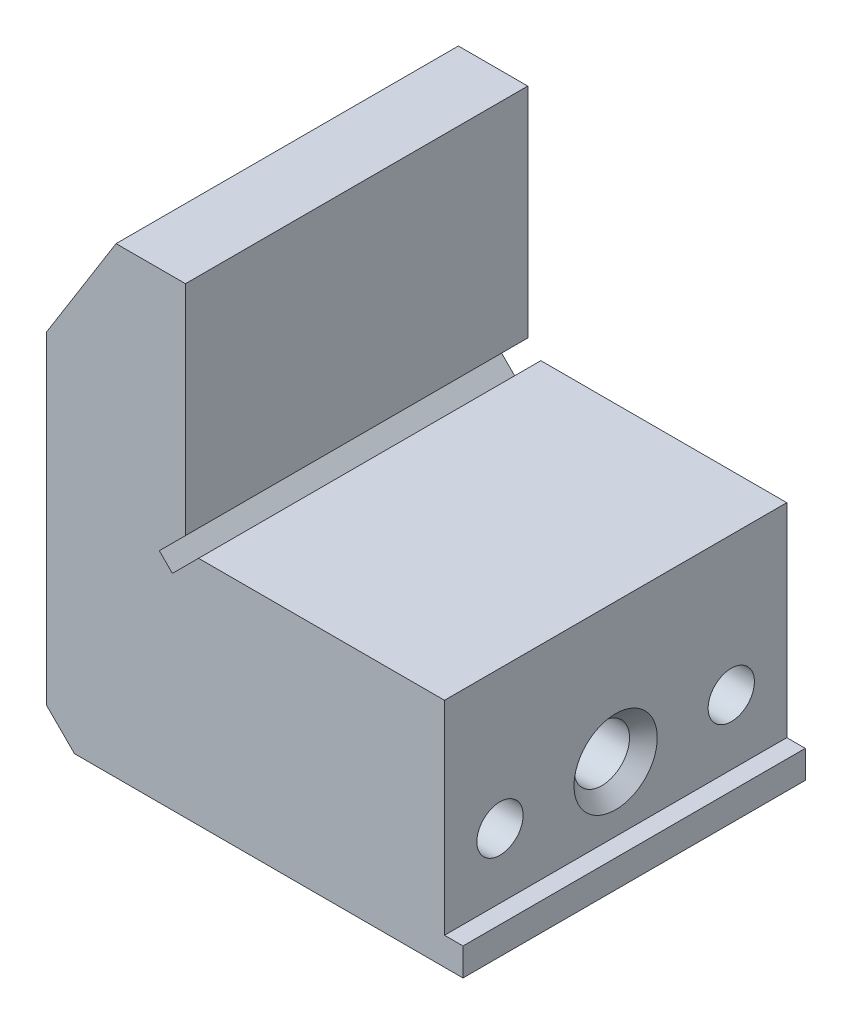
ISO-10303-21;
HEADER;
FILE_DESCRIPTION(('STEP AP214'),'2;1');
FILE_NAME('part.step','',(''),(''),'','','');
FILE_SCHEMA(('AUTOMOTIVE_DESIGN { 1 0 10303 214 1 1 1 1 }'));
ENDSEC;
DATA;
#1=APPLICATION_CONTEXT('core data for automotive mechanical design processes');
#2=APPLICATION_PROTOCOL_DEFINITION('international standard','automotive_design',2000,#1);
#3=PRODUCT_CONTEXT('',#1,'mechanical');
#4=PRODUCT('Part','Part','',(#3));
#5=PRODUCT_RELATED_PRODUCT_CATEGORY('part','',(#4));
#6=PRODUCT_DEFINITION_FORMATION('','',#4);
#7=PRODUCT_DEFINITION_CONTEXT('part definition',#1,'design');
#8=PRODUCT_DEFINITION('design','',#6,#7);
#9=PRODUCT_DEFINITION_SHAPE('','',#8);
#10=(LENGTH_UNIT() NAMED_UNIT(*) SI_UNIT(.MILLI.,.METRE.));
#11=(NAMED_UNIT(*) PLANE_ANGLE_UNIT() SI_UNIT($,.RADIAN.));
#12=(NAMED_UNIT(*) SI_UNIT($,.STERADIAN.) SOLID_ANGLE_UNIT());
#13=UNCERTAINTY_MEASURE_WITH_UNIT(LENGTH_MEASURE(1.E-05),#10,'distance_accuracy_value','');
#14=(GEOMETRIC_REPRESENTATION_CONTEXT(3) GLOBAL_UNCERTAINTY_ASSIGNED_CONTEXT((#13)) GLOBAL_UNIT_ASSIGNED_CONTEXT((#10,
#11,#12)) REPRESENTATION_CONTEXT('',''));
#15=CARTESIAN_POINT('',(0.,0.,0.));
#16=DIRECTION('',(0.,0.,1.));
#17=DIRECTION('',(1.,0.,0.));
#18=AXIS2_PLACEMENT_3D('',#15,#16,#17);
#19=CARTESIAN_POINT('',(3.,-25.,18.5));
#20=DIRECTION('',(0.707106781186548,0.707106781186547,0.));
#21=DIRECTION('',(0.,0.,-1.));
#22=AXIS2_PLACEMENT_3D('',#19,#20,#21);
#23=PLANE('',#22);
#24=DIRECTION('',(-0.707106781186547,0.707106781186548,0.));
#25=VECTOR('',#24,1.);
#26=CARTESIAN_POINT('',(3.00000000000001,-25.,-12.));
#27=LINE('',#26,#25);
#28=CARTESIAN_POINT('',(0.,-22.,-12.));
#29=VERTEX_POINT('',#28);
#30=CARTESIAN_POINT('',(3.00000000000001,-25.,-12.));
#31=VERTEX_POINT('',#30);
#32=EDGE_CURVE('E12',#29,#31,#27,.F.);
#33=ORIENTED_EDGE('',*,*,#32,.F.);
#34=DIRECTION('',(0.,0.,1.));
#35=VECTOR('',#34,1.);
#36=CARTESIAN_POINT('',(0.,-22.,18.5));
#37=LINE('',#36,#35);
#38=CARTESIAN_POINT('',(0.,-22.,-18.5));
#39=VERTEX_POINT('',#38);
#40=EDGE_CURVE('E318',#39,#29,#37,.T.);
#41=ORIENTED_EDGE('',*,*,#40,.F.);
#42=DIRECTION('',(0.707106781186547,-0.707106781186548,0.));
#43=VECTOR('',#42,1.);
#44=CARTESIAN_POINT('',(-11.,-11.,-18.5));
#45=LINE('',#44,#43);
#46=CARTESIAN_POINT('',(3.00000000000002,-25.,-18.5));
#47=VERTEX_POINT('',#46);
#48=EDGE_CURVE('E312',#47,#39,#45,.F.);
#49=ORIENTED_EDGE('',*,*,#48,.F.);
#50=DIRECTION('',(0.,0.,-1.));
#51=VECTOR('',#50,1.);
#52=CARTESIAN_POINT('',(3.,-25.,18.5));
#53=LINE('',#52,#51);
#54=EDGE_CURVE('E313',#31,#47,#53,.T.);
#55=ORIENTED_EDGE('',*,*,#54,.F.);
#56=EDGE_LOOP('',(#33,#41,#49,#55));
#57=FACE_BOUND('',#56,.T.);
#58=ADVANCED_FACE('F43',(#57),#23,.F.);
#59=CARTESIAN_POINT('',(45.,-25.,18.5));
#60=DIRECTION('',(0.,1.,0.));
#61=DIRECTION('',(-1.,0.,0.));
#62=AXIS2_PLACEMENT_3D('',#59,#60,#61);
#63=PLANE('',#62);
#64=DIRECTION('',(0.,0.,-1.));
#65=VECTOR('',#64,1.);
#66=CARTESIAN_POINT('',(27.,-25.,-12.));
#67=LINE('',#66,#65);
#68=CARTESIAN_POINT('',(27.,-25.,12.));
#69=VERTEX_POINT('',#68);
#70=CARTESIAN_POINT('',(27.,-25.,-12.));
#71=VERTEX_POINT('',#70);
#72=EDGE_CURVE('E206',#69,#71,#67,.T.);
#73=ORIENTED_EDGE('',*,*,#72,.T.);
#74=DIRECTION('',(-1.,0.,0.));
#75=VECTOR('',#74,1.);
#76=CARTESIAN_POINT('',(75.,-25.,-12.));
#77=LINE('',#76,#75);
#78=EDGE_CURVE('E204',#71,#31,#77,.T.);
#79=ORIENTED_EDGE('',*,*,#78,.T.);
#80=ORIENTED_EDGE('',*,*,#54,.T.);
#81=DIRECTION('',(1.,0.,0.));
#82=VECTOR('',#81,1.);
#83=CARTESIAN_POINT('',(45.,-25.,-18.5));
#84=LINE('',#83,#82);
#85=CARTESIAN_POINT('',(45.,-25.,-18.5));
#86=VERTEX_POINT('',#85);
#87=EDGE_CURVE('E245',#47,#86,#84,.T.);
#88=ORIENTED_EDGE('',*,*,#87,.T.);
#89=DIRECTION('',(0.,0.,-1.));
#90=VECTOR('',#89,1.);
#91=CARTESIAN_POINT('',(45.,-25.,18.5));
#92=LINE('',#91,#90);
#93=CARTESIAN_POINT('',(45.,-25.,18.5));
#94=VERTEX_POINT('',#93);
#95=EDGE_CURVE('E306',#94,#86,#92,.T.);
#96=ORIENTED_EDGE('',*,*,#95,.F.);
#97=DIRECTION('',(1.,0.,0.));
#98=VECTOR('',#97,1.);
#99=CARTESIAN_POINT('',(45.,-25.,18.5));
#100=LINE('',#99,#98);
#101=CARTESIAN_POINT('',(3.00000000000002,-25.,18.5));
#102=VERTEX_POINT('',#101);
#103=EDGE_CURVE('E251',#102,#94,#100,.T.);
#104=ORIENTED_EDGE('',*,*,#103,.F.);
#105=CARTESIAN_POINT('',(3.,-25.,12.));
#106=VERTEX_POINT('',#105);
#107=EDGE_CURVE('E315',#102,#106,#53,.T.);
#108=ORIENTED_EDGE('',*,*,#107,.T.);
#109=DIRECTION('',(-1.,0.,0.));
#110=VECTOR('',#109,1.);
#111=CARTESIAN_POINT('',(75.,-25.,12.));
#112=LINE('',#111,#110);
#113=EDGE_CURVE('E58',#69,#106,#112,.T.);
#114=ORIENTED_EDGE('',*,*,#113,.F.);
#115=EDGE_LOOP('',(#73,#79,#80,#88,#96,#104,#108,#114));
#116=FACE_BOUND('',#115,.T.);
#117=ADVANCED_FACE('F336',(#116),#63,.F.);
#118=CARTESIAN_POINT('',(45.,-22.,18.5));
#119=DIRECTION('',(-1.,0.,0.));
#120=DIRECTION('',(0.,0.,1.));
#121=AXIS2_PLACEMENT_3D('',#118,#119,#120);
#122=PLANE('',#121);
#123=DIRECTION('',(0.,1.,0.));
#124=VECTOR('',#123,1.);
#125=CARTESIAN_POINT('',(45.,-22.,-18.5));
#126=LINE('',#125,#124);
#127=CARTESIAN_POINT('',(45.,-22.,-18.5));
#128=VERTEX_POINT('',#127);
#129=EDGE_CURVE('E273',#86,#128,#126,.T.);
#130=ORIENTED_EDGE('',*,*,#129,.T.);
#131=DIRECTION('',(0.,0.,-1.));
#132=VECTOR('',#131,1.);
#133=CARTESIAN_POINT('',(45.,-22.,18.5));
#134=LINE('',#133,#132);
#135=CARTESIAN_POINT('',(45.,-22.,18.5));
#136=VERTEX_POINT('',#135);
#137=EDGE_CURVE('E303',#136,#128,#134,.T.);
#138=ORIENTED_EDGE('',*,*,#137,.F.);
#139=DIRECTION('',(0.,1.,0.));
#140=VECTOR('',#139,1.);
#141=CARTESIAN_POINT('',(45.,-22.,18.5));
#142=LINE('',#141,#140);
#143=EDGE_CURVE('E258',#94,#136,#142,.T.);
#144=ORIENTED_EDGE('',*,*,#143,.F.);
#145=ORIENTED_EDGE('',*,*,#95,.T.);
#146=EDGE_LOOP('',(#130,#138,#144,#145));
#147=FACE_BOUND('',#146,.T.);
#148=ADVANCED_FACE('F347',(#147),#122,.F.);
#149=CARTESIAN_POINT('',(43.,-22.,18.5));
#150=DIRECTION('',(0.,-1.,0.));
#151=DIRECTION('',(0.,0.,-1.));
#152=AXIS2_PLACEMENT_3D('',#149,#150,#151);
#153=PLANE('',#152);
#154=DIRECTION('',(-1.,0.,0.));
#155=VECTOR('',#154,1.);
#156=CARTESIAN_POINT('',(43.,-22.,-18.5));
#157=LINE('',#156,#155);
#158=CARTESIAN_POINT('',(43.,-22.,-18.5));
#159=VERTEX_POINT('',#158);
#160=EDGE_CURVE('E277',#128,#159,#157,.T.);
#161=ORIENTED_EDGE('',*,*,#160,.T.);
#162=DIRECTION('',(0.,0.,-1.));
#163=VECTOR('',#162,1.);
#164=CARTESIAN_POINT('',(43.,-22.,18.5));
#165=LINE('',#164,#163);
#166=CARTESIAN_POINT('',(43.,-22.,18.5));
#167=VERTEX_POINT('',#166);
#168=EDGE_CURVE('E304',#167,#159,#165,.T.);
#169=ORIENTED_EDGE('',*,*,#168,.F.);
#170=DIRECTION('',(-1.,0.,0.));
#171=VECTOR('',#170,1.);
#172=CARTESIAN_POINT('',(43.,-22.,18.5));
#173=LINE('',#172,#171);
#174=EDGE_CURVE('E256',#136,#167,#173,.T.);
#175=ORIENTED_EDGE('',*,*,#174,.F.);
#176=ORIENTED_EDGE('',*,*,#137,.T.);
#177=EDGE_LOOP('',(#161,#169,#175,#176));
#178=FACE_BOUND('',#177,.T.);
#179=ADVANCED_FACE('F354',(#178),#153,.F.);
#180=CARTESIAN_POINT('',(43.,0.,18.5));
#181=DIRECTION('',(-1.,0.,0.));
#182=DIRECTION('',(0.,0.,1.));
#183=AXIS2_PLACEMENT_3D('',#180,#181,#182);
#184=PLANE('',#183);
#185=CARTESIAN_POINT('',(43.,-15.,-12.5));
#186=DIRECTION('',(1.,0.,0.));
#187=DIRECTION('',(0.,0.,-1.));
#188=AXIS2_PLACEMENT_3D('',#185,#186,#187);
#189=CIRCLE('',#188,2.49999999999999);
#190=CARTESIAN_POINT('',(43.,-15.,-15.));
#191=VERTEX_POINT('',#190);
#192=EDGE_CURVE('E183',#191,#191,#189,.T.);
#193=ORIENTED_EDGE('',*,*,#192,.F.);
#194=EDGE_LOOP('',(#193));
#195=FACE_BOUND('',#194,.T.);
#196=CARTESIAN_POINT('',(43.,-15.,12.5));
#197=DIRECTION('',(1.,0.,0.));
#198=DIRECTION('',(0.,0.,-1.));
#199=AXIS2_PLACEMENT_3D('',#196,#197,#198);
#200=CIRCLE('',#199,2.49999999999999);
#201=CARTESIAN_POINT('',(43.,-15.,10.));
#202=VERTEX_POINT('',#201);
#203=EDGE_CURVE('E184',#202,#202,#200,.T.);
#204=ORIENTED_EDGE('',*,*,#203,.F.);
#205=EDGE_LOOP('',(#204));
#206=FACE_BOUND('',#205,.T.);
#207=CARTESIAN_POINT('',(43.,-15.,0.));
#208=DIRECTION('',(1.,0.,0.));
#209=DIRECTION('',(0.,0.,-1.));
#210=AXIS2_PLACEMENT_3D('',#207,#208,#209);
#211=CIRCLE('',#210,4.5);
#212=CARTESIAN_POINT('',(43.,-15.,-4.5));
#213=VERTEX_POINT('',#212);
#214=EDGE_CURVE('E193',#213,#213,#211,.T.);
#215=ORIENTED_EDGE('',*,*,#214,.F.);
#216=EDGE_LOOP('',(#215));
#217=FACE_BOUND('',#216,.T.);
#218=DIRECTION('',(0.,1.,0.));
#219=VECTOR('',#218,1.);
#220=CARTESIAN_POINT('',(43.,0.,-18.5));
#221=LINE('',#220,#219);
#222=CARTESIAN_POINT('',(43.,0.,-18.5));
#223=VERTEX_POINT('',#222);
#224=EDGE_CURVE('E279',#159,#223,#221,.T.);
#225=ORIENTED_EDGE('',*,*,#224,.T.);
#226=DIRECTION('',(0.,0.,-1.));
#227=VECTOR('',#226,1.);
#228=CARTESIAN_POINT('',(43.,0.,18.5));
#229=LINE('',#228,#227);
#230=CARTESIAN_POINT('',(43.,0.,18.5));
#231=VERTEX_POINT('',#230);
#232=EDGE_CURVE('E300',#231,#223,#229,.T.);
#233=ORIENTED_EDGE('',*,*,#232,.F.);
#234=DIRECTION('',(0.,1.,0.));
#235=VECTOR('',#234,1.);
#236=CARTESIAN_POINT('',(43.,0.,18.5));
#237=LINE('',#236,#235);
#238=EDGE_CURVE('E257',#167,#231,#237,.T.);
#239=ORIENTED_EDGE('',*,*,#238,.F.);
#240=ORIENTED_EDGE('',*,*,#168,.T.);
#241=EDGE_LOOP('',(#225,#233,#239,#240));
#242=FACE_BOUND('',#241,.T.);
#243=ADVANCED_FACE('F357',(#195,#206,#217,#242),#184,.F.);
#244=CARTESIAN_POINT('',(15.,0.,18.5));
#245=DIRECTION('',(0.,-1.,0.));
#246=DIRECTION('',(0.,0.,-1.));
#247=AXIS2_PLACEMENT_3D('',#244,#245,#246);
#248=PLANE('',#247);
#249=DIRECTION('',(-1.,0.,0.));
#250=VECTOR('',#249,1.);
#251=CARTESIAN_POINT('',(15.,0.,-18.5));
#252=LINE('',#251,#250);
#253=CARTESIAN_POINT('',(16.4142135623731,0.,-18.5));
#254=VERTEX_POINT('',#253);
#255=EDGE_CURVE('E278',#223,#254,#252,.T.);
#256=ORIENTED_EDGE('',*,*,#255,.T.);
#257=DIRECTION('',(0.,0.,1.));
#258=VECTOR('',#257,1.);
#259=CARTESIAN_POINT('',(16.4142135623731,0.,-18.5));
#260=LINE('',#259,#258);
#261=CARTESIAN_POINT('',(16.4142135623731,0.,18.5));
#262=VERTEX_POINT('',#261);
#263=EDGE_CURVE('E70',#254,#262,#260,.T.);
#264=ORIENTED_EDGE('',*,*,#263,.T.);
#265=DIRECTION('',(-1.,0.,0.));
#266=VECTOR('',#265,1.);
#267=CARTESIAN_POINT('',(15.,0.,18.5));
#268=LINE('',#267,#266);
#269=EDGE_CURVE('E265',#231,#262,#268,.T.);
#270=ORIENTED_EDGE('',*,*,#269,.F.);
#271=ORIENTED_EDGE('',*,*,#232,.T.);
#272=EDGE_LOOP('',(#256,#264,#270,#271));
#273=FACE_BOUND('',#272,.T.);
#274=ADVANCED_FACE('F358',(#273),#248,.F.);
#275=CARTESIAN_POINT('',(15.,25.,18.5));
#276=DIRECTION('',(-1.,0.,0.));
#277=DIRECTION('',(0.,-1.,0.));
#278=AXIS2_PLACEMENT_3D('',#275,#276,#277);
#279=PLANE('',#278);
#280=DIRECTION('',(0.,1.,0.));
#281=VECTOR('',#280,1.);
#282=CARTESIAN_POINT('',(15.,25.,18.5));
#283=LINE('',#282,#281);
#284=CARTESIAN_POINT('',(15.,1.4142135623731,18.5));
#285=VERTEX_POINT('',#284);
#286=CARTESIAN_POINT('',(15.,25.,18.5));
#287=VERTEX_POINT('',#286);
#288=EDGE_CURVE('E264',#285,#287,#283,.T.);
#289=ORIENTED_EDGE('',*,*,#288,.F.);
#290=DIRECTION('',(0.,0.,1.));
#291=VECTOR('',#290,1.);
#292=CARTESIAN_POINT('',(15.,1.4142135623731,-18.5));
#293=LINE('',#292,#291);
#294=CARTESIAN_POINT('',(15.,1.4142135623731,-18.5));
#295=VERTEX_POINT('',#294);
#296=EDGE_CURVE('E241',#295,#285,#293,.T.);
#297=ORIENTED_EDGE('',*,*,#296,.F.);
#298=DIRECTION('',(0.,1.,0.));
#299=VECTOR('',#298,1.);
#300=CARTESIAN_POINT('',(15.,25.,-18.5));
#301=LINE('',#300,#299);
#302=CARTESIAN_POINT('',(15.,25.,-18.5));
#303=VERTEX_POINT('',#302);
#304=EDGE_CURVE('E282',#295,#303,#301,.T.);
#305=ORIENTED_EDGE('',*,*,#304,.T.);
#306=DIRECTION('',(0.,0.,-1.));
#307=VECTOR('',#306,1.);
#308=CARTESIAN_POINT('',(15.,25.,18.5));
#309=LINE('',#308,#307);
#310=EDGE_CURVE('E298',#287,#303,#309,.T.);
#311=ORIENTED_EDGE('',*,*,#310,.F.);
#312=EDGE_LOOP('',(#289,#297,#305,#311));
#313=FACE_BOUND('',#312,.T.);
#314=ADVANCED_FACE('F373',(#313),#279,.F.);
#315=CARTESIAN_POINT('',(7.49843222291195,25.,18.5));
#316=DIRECTION('',(0.,-1.,0.));
#317=DIRECTION('',(0.,0.,-1.));
#318=AXIS2_PLACEMENT_3D('',#315,#316,#317);
#319=PLANE('',#318);
#320=DIRECTION('',(-1.,0.,0.));
#321=VECTOR('',#320,1.);
#322=CARTESIAN_POINT('',(7.49843222291195,25.,-18.5));
#323=LINE('',#322,#321);
#324=CARTESIAN_POINT('',(7.49843222291195,25.,-18.5));
#325=VERTEX_POINT('',#324);
#326=EDGE_CURVE('E281',#303,#325,#323,.T.);
#327=ORIENTED_EDGE('',*,*,#326,.T.);
#328=DIRECTION('',(0.,0.,-1.));
#329=VECTOR('',#328,1.);
#330=CARTESIAN_POINT('',(7.49843222291195,25.,18.5));
#331=LINE('',#330,#329);
#332=CARTESIAN_POINT('',(7.49843222291195,25.,18.5));
#333=VERTEX_POINT('',#332);
#334=EDGE_CURVE('E291',#333,#325,#331,.T.);
#335=ORIENTED_EDGE('',*,*,#334,.F.);
#336=DIRECTION('',(-1.,0.,0.));
#337=VECTOR('',#336,1.);
#338=CARTESIAN_POINT('',(7.49843222291195,25.,18.5));
#339=LINE('',#338,#337);
#340=EDGE_CURVE('E270',#287,#333,#339,.T.);
#341=ORIENTED_EDGE('',*,*,#340,.F.);
#342=ORIENTED_EDGE('',*,*,#310,.T.);
#343=EDGE_LOOP('',(#327,#335,#341,#342));
#344=FACE_BOUND('',#343,.T.);
#345=ADVANCED_FACE('F377',(#344),#319,.F.);
#346=CARTESIAN_POINT('',(0.,13.,18.5));
#347=DIRECTION('',(0.848048096156426,-0.529919264233206,0.));
#348=DIRECTION('',(0.529919264233206,0.848048096156425,0.));
#349=AXIS2_PLACEMENT_3D('',#346,#347,#348);
#350=PLANE('',#349);
#351=DIRECTION('',(-0.529919264233206,-0.848048096156425,0.));
#352=VECTOR('',#351,1.);
#353=CARTESIAN_POINT('',(0.,13.,-18.5));
#354=LINE('',#353,#352);
#355=CARTESIAN_POINT('',(0.,13.,-18.5));
#356=VERTEX_POINT('',#355);
#357=EDGE_CURVE('E289',#325,#356,#354,.T.);
#358=ORIENTED_EDGE('',*,*,#357,.T.);
#359=DIRECTION('',(0.,0.,-1.));
#360=VECTOR('',#359,1.);
#361=CARTESIAN_POINT('',(0.,13.,18.5));
#362=LINE('',#361,#360);
#363=CARTESIAN_POINT('',(0.,13.,18.5));
#364=VERTEX_POINT('',#363);
#365=EDGE_CURVE('E275',#364,#356,#362,.T.);
#366=ORIENTED_EDGE('',*,*,#365,.F.);
#367=DIRECTION('',(-0.529919264233206,-0.848048096156425,0.));
#368=VECTOR('',#367,1.);
#369=CARTESIAN_POINT('',(0.,13.,18.5));
#370=LINE('',#369,#368);
#371=EDGE_CURVE('E267',#333,#364,#370,.T.);
#372=ORIENTED_EDGE('',*,*,#371,.F.);
#373=ORIENTED_EDGE('',*,*,#334,.T.);
#374=EDGE_LOOP('',(#358,#366,#372,#373));
#375=FACE_BOUND('',#374,.T.);
#376=ADVANCED_FACE('F382',(#375),#350,.F.);
#377=CARTESIAN_POINT('',(0.,0.,18.5));
#378=DIRECTION('',(1.,0.,0.));
#379=DIRECTION('',(0.,0.,-1.));
#380=AXIS2_PLACEMENT_3D('',#377,#378,#379);
#381=PLANE('',#380);
#382=ORIENTED_EDGE('',*,*,#40,.T.);
#383=DIRECTION('',(0.,-1.,0.));
#384=VECTOR('',#383,1.);
#385=CARTESIAN_POINT('',(0.,-25.,-12.));
#386=LINE('',#385,#384);
#387=CARTESIAN_POINT('',(0.,-10.0682878005387,-12.));
#388=VERTEX_POINT('',#387);
#389=EDGE_CURVE('E214',#388,#29,#386,.T.);
#390=ORIENTED_EDGE('',*,*,#389,.F.);
#391=CARTESIAN_POINT('',(0.,-32.,0.));
#392=DIRECTION('',(-1.,0.,0.));
#393=DIRECTION('',(0.,0.,-1.));
#394=AXIS2_PLACEMENT_3D('',#391,#392,#393);
#395=CIRCLE('',#394,25.);
#396=CARTESIAN_POINT('',(0.,-10.0682878005387,12.));
#397=VERTEX_POINT('',#396);
#398=EDGE_CURVE('E215',#397,#388,#395,.T.);
#399=ORIENTED_EDGE('',*,*,#398,.F.);
#400=DIRECTION('',(0.,1.,0.));
#401=VECTOR('',#400,1.);
#402=CARTESIAN_POINT('',(0.,-10.0682878005387,12.));
#403=LINE('',#402,#401);
#404=CARTESIAN_POINT('',(0.,-22.,12.));
#405=VERTEX_POINT('',#404);
#406=EDGE_CURVE('E209',#405,#397,#403,.T.);
#407=ORIENTED_EDGE('',*,*,#406,.F.);
#408=CARTESIAN_POINT('',(0.,-22.,18.5));
#409=VERTEX_POINT('',#408);
#410=EDGE_CURVE('E320',#405,#409,#37,.T.);
#411=ORIENTED_EDGE('',*,*,#410,.T.);
#412=DIRECTION('',(0.,-1.,0.));
#413=VECTOR('',#412,1.);
#414=CARTESIAN_POINT('',(0.,-25.,18.5));
#415=LINE('',#414,#413);
#416=EDGE_CURVE('E248',#364,#409,#415,.T.);
#417=ORIENTED_EDGE('',*,*,#416,.F.);
#418=ORIENTED_EDGE('',*,*,#365,.T.);
#419=DIRECTION('',(0.,-1.,0.));
#420=VECTOR('',#419,1.);
#421=CARTESIAN_POINT('',(0.,0.,-18.5));
#422=LINE('',#421,#420);
#423=EDGE_CURVE('E255',#356,#39,#422,.T.);
#424=ORIENTED_EDGE('',*,*,#423,.T.);
#425=EDGE_LOOP('',(#382,#390,#399,#407,#411,#417,#418,#424));
#426=FACE_BOUND('',#425,.T.);
#427=ADVANCED_FACE('F332',(#426),#381,.F.);
#428=CARTESIAN_POINT('',(0.,0.,18.5));
#429=DIRECTION('',(0.,0.,-1.));
#430=DIRECTION('',(-1.,0.,0.));
#431=AXIS2_PLACEMENT_3D('',#428,#429,#430);
#432=PLANE('',#431);
#433=DIRECTION('',(0.707106781186548,-0.707106781186547,0.));
#434=VECTOR('',#433,1.);
#435=CARTESIAN_POINT('',(12.8786796564404,-2.12132034355965,18.5));
#436=LINE('',#435,#434);
#437=CARTESIAN_POINT('',(12.1715728752538,-1.4142135623731,18.5));
#438=VERTEX_POINT('',#437);
#439=CARTESIAN_POINT('',(13.5857864376269,-2.82842712474619,18.5));
#440=VERTEX_POINT('',#439);
#441=EDGE_CURVE('E232',#438,#440,#436,.T.);
#442=ORIENTED_EDGE('',*,*,#441,.F.);
#443=DIRECTION('',(-0.707106781186546,-0.707106781186549,0.));
#444=VECTOR('',#443,1.);
#445=CARTESIAN_POINT('',(12.1715728752538,-1.4142135623731,18.5));
#446=LINE('',#445,#444);
#447=EDGE_CURVE('E236',#285,#438,#446,.T.);
#448=ORIENTED_EDGE('',*,*,#447,.F.);
#449=ORIENTED_EDGE('',*,*,#288,.T.);
#450=ORIENTED_EDGE('',*,*,#340,.T.);
#451=ORIENTED_EDGE('',*,*,#371,.T.);
#452=ORIENTED_EDGE('',*,*,#416,.T.);
#453=DIRECTION('',(-0.707106781186547,0.707106781186548,0.));
#454=VECTOR('',#453,1.);
#455=CARTESIAN_POINT('',(3.,-25.,18.5));
#456=LINE('',#455,#454);
#457=EDGE_CURVE('E321',#409,#102,#456,.F.);
#458=ORIENTED_EDGE('',*,*,#457,.T.);
#459=ORIENTED_EDGE('',*,*,#103,.T.);
#460=ORIENTED_EDGE('',*,*,#143,.T.);
#461=ORIENTED_EDGE('',*,*,#174,.T.);
#462=ORIENTED_EDGE('',*,*,#238,.T.);
#463=ORIENTED_EDGE('',*,*,#269,.T.);
#464=DIRECTION('',(0.707106781186547,0.707106781186549,0.));
#465=VECTOR('',#464,1.);
#466=CARTESIAN_POINT('',(16.4142135623731,0.,18.5));
#467=LINE('',#466,#465);
#468=EDGE_CURVE('E228',#440,#262,#467,.T.);
#469=ORIENTED_EDGE('',*,*,#468,.F.);
#470=EDGE_LOOP('',(#442,#448,#449,#450,#451,#452,#458,#459,#460,#461,#462,#463,#469));
#471=FACE_BOUND('',#470,.T.);
#472=ADVANCED_FACE('F339',(#471),#432,.F.);
#473=CARTESIAN_POINT('',(0.,0.,-18.5));
#474=DIRECTION('',(0.,0.,-1.));
#475=DIRECTION('',(-1.,0.,0.));
#476=AXIS2_PLACEMENT_3D('',#473,#474,#475);
#477=PLANE('',#476);
#478=DIRECTION('',(-0.707106781186546,-0.707106781186549,0.));
#479=VECTOR('',#478,1.);
#480=CARTESIAN_POINT('',(12.1715728752538,-1.4142135623731,-18.5));
#481=LINE('',#480,#479);
#482=CARTESIAN_POINT('',(12.1715728752538,-1.4142135623731,-18.5));
#483=VERTEX_POINT('',#482);
#484=EDGE_CURVE('E235',#295,#483,#481,.T.);
#485=ORIENTED_EDGE('',*,*,#484,.T.);
#486=DIRECTION('',(0.707106781186547,-0.707106781186547,0.));
#487=VECTOR('',#486,1.);
#488=CARTESIAN_POINT('',(13.5857864376269,-2.82842712474619,-18.5));
#489=LINE('',#488,#487);
#490=CARTESIAN_POINT('',(13.5857864376269,-2.82842712474619,-18.5));
#491=VERTEX_POINT('',#490);
#492=EDGE_CURVE('E229',#483,#491,#489,.T.);
#493=ORIENTED_EDGE('',*,*,#492,.T.);
#494=DIRECTION('',(0.707106781186547,0.707106781186549,0.));
#495=VECTOR('',#494,1.);
#496=CARTESIAN_POINT('',(16.4142135623731,0.,-18.5));
#497=LINE('',#496,#495);
#498=EDGE_CURVE('E226',#491,#254,#497,.T.);
#499=ORIENTED_EDGE('',*,*,#498,.T.);
#500=ORIENTED_EDGE('',*,*,#255,.F.);
#501=ORIENTED_EDGE('',*,*,#224,.F.);
#502=ORIENTED_EDGE('',*,*,#160,.F.);
#503=ORIENTED_EDGE('',*,*,#129,.F.);
#504=ORIENTED_EDGE('',*,*,#87,.F.);
#505=ORIENTED_EDGE('',*,*,#48,.T.);
#506=ORIENTED_EDGE('',*,*,#423,.F.);
#507=ORIENTED_EDGE('',*,*,#357,.F.);
#508=ORIENTED_EDGE('',*,*,#326,.F.);
#509=ORIENTED_EDGE('',*,*,#304,.F.);
#510=EDGE_LOOP('',(#485,#493,#499,#500,#501,#502,#503,#504,#505,#506,#507,#508,#509));
#511=FACE_BOUND('',#510,.T.);
#512=ADVANCED_FACE('F389',(#511),#477,.T.);
#513=DIRECTION('',(0.707106781186547,-0.707106781186548,0.));
#514=VECTOR('',#513,1.);
#515=CARTESIAN_POINT('',(3.,-25.,12.));
#516=LINE('',#515,#514);
#517=EDGE_CURVE('E52',#106,#405,#516,.F.);
#518=ORIENTED_EDGE('',*,*,#517,.F.);
#519=ORIENTED_EDGE('',*,*,#107,.F.);
#520=ORIENTED_EDGE('',*,*,#457,.F.);
#521=ORIENTED_EDGE('',*,*,#410,.F.);
#522=EDGE_LOOP('',(#518,#519,#520,#521));
#523=FACE_BOUND('',#522,.T.);
#524=ADVANCED_FACE('F46',(#523),#23,.F.);
#525=CARTESIAN_POINT('',(12.8786796564404,-2.12132034355965,-18.5));
#526=DIRECTION('',(-0.707106781186547,-0.707106781186548,0.));
#527=DIRECTION('',(0.707106781186548,-0.707106781186547,0.));
#528=AXIS2_PLACEMENT_3D('',#525,#526,#527);
#529=PLANE('',#528);
#530=ORIENTED_EDGE('',*,*,#441,.T.);
#531=DIRECTION('',(0.,0.,1.));
#532=VECTOR('',#531,1.);
#533=CARTESIAN_POINT('',(13.5857864376269,-2.82842712474619,-18.5));
#534=LINE('',#533,#532);
#535=EDGE_CURVE('E237',#491,#440,#534,.T.);
#536=ORIENTED_EDGE('',*,*,#535,.F.);
#537=ORIENTED_EDGE('',*,*,#492,.F.);
#538=DIRECTION('',(0.,0.,1.));
#539=VECTOR('',#538,1.);
#540=CARTESIAN_POINT('',(12.1715728752538,-1.4142135623731,-18.5));
#541=LINE('',#540,#539);
#542=EDGE_CURVE('E244',#483,#438,#541,.T.);
#543=ORIENTED_EDGE('',*,*,#542,.T.);
#544=EDGE_LOOP('',(#530,#536,#537,#543));
#545=FACE_BOUND('',#544,.T.);
#546=ADVANCED_FACE('F364',(#545),#529,.F.);
#547=CARTESIAN_POINT('',(12.1715728752538,-1.4142135623731,-18.5));
#548=DIRECTION('',(-0.707106781186549,0.707106781186546,0.));
#549=DIRECTION('',(-0.707106781186546,-0.707106781186549,0.));
#550=AXIS2_PLACEMENT_3D('',#547,#548,#549);
#551=PLANE('',#550);
#552=ORIENTED_EDGE('',*,*,#447,.T.);
#553=ORIENTED_EDGE('',*,*,#542,.F.);
#554=ORIENTED_EDGE('',*,*,#484,.F.);
#555=ORIENTED_EDGE('',*,*,#296,.T.);
#556=EDGE_LOOP('',(#552,#553,#554,#555));
#557=FACE_BOUND('',#556,.T.);
#558=ADVANCED_FACE('F366',(#557),#551,.F.);
#559=CARTESIAN_POINT('',(16.4142135623731,0.,-18.5));
#560=DIRECTION('',(0.707106781186549,-0.707106781186547,0.));
#561=DIRECTION('',(0.707106781186547,0.707106781186549,0.));
#562=AXIS2_PLACEMENT_3D('',#559,#560,#561);
#563=PLANE('',#562);
#564=ORIENTED_EDGE('',*,*,#468,.T.);
#565=ORIENTED_EDGE('',*,*,#263,.F.);
#566=ORIENTED_EDGE('',*,*,#498,.F.);
#567=ORIENTED_EDGE('',*,*,#535,.T.);
#568=EDGE_LOOP('',(#564,#565,#566,#567));
#569=FACE_BOUND('',#568,.T.);
#570=ADVANCED_FACE('F361',(#569),#563,.F.);
#571=CARTESIAN_POINT('',(75.,-25.,-12.));
#572=DIRECTION('',(0.,0.,-1.));
#573=DIRECTION('',(0.,1.,0.));
#574=AXIS2_PLACEMENT_3D('',#571,#572,#573);
#575=PLANE('',#574);
#576=ORIENTED_EDGE('',*,*,#32,.T.);
#577=ORIENTED_EDGE('',*,*,#78,.F.);
#578=DIRECTION('',(0.,1.,0.));
#579=VECTOR('',#578,1.);
#580=CARTESIAN_POINT('',(27.,-25.,-12.));
#581=LINE('',#580,#579);
#582=CARTESIAN_POINT('',(27.,-10.0682878005387,-12.));
#583=VERTEX_POINT('',#582);
#584=EDGE_CURVE('E201',#71,#583,#581,.T.);
#585=ORIENTED_EDGE('',*,*,#584,.T.);
#586=DIRECTION('',(-1.,0.,0.));
#587=VECTOR('',#586,1.);
#588=CARTESIAN_POINT('',(75.,-10.0682878005387,-12.));
#589=LINE('',#588,#587);
#590=EDGE_CURVE('E218',#583,#388,#589,.T.);
#591=ORIENTED_EDGE('',*,*,#590,.T.);
#592=ORIENTED_EDGE('',*,*,#389,.T.);
#593=EDGE_LOOP('',(#576,#577,#585,#591,#592));
#594=FACE_BOUND('',#593,.T.);
#595=ADVANCED_FACE('F395',(#594),#575,.F.);
#596=CARTESIAN_POINT('',(75.,-32.,0.));
#597=DIRECTION('',(-1.,0.,0.));
#598=DIRECTION('',(0.,0.,1.));
#599=AXIS2_PLACEMENT_3D('',#596,#597,#598);
#600=CYLINDRICAL_SURFACE('',#599,25.);
#601=CARTESIAN_POINT('',(27.,-32.,0.));
#602=DIRECTION('',(-1.,0.,0.));
#603=DIRECTION('',(0.,0.,1.));
#604=AXIS2_PLACEMENT_3D('',#601,#602,#603);
#605=CIRCLE('',#604,25.);
#606=CARTESIAN_POINT('',(27.,-10.0682878005387,12.));
#607=VERTEX_POINT('',#606);
#608=EDGE_CURVE('E203',#583,#607,#605,.F.);
#609=ORIENTED_EDGE('',*,*,#608,.T.);
#610=DIRECTION('',(-1.,0.,0.));
#611=VECTOR('',#610,1.);
#612=CARTESIAN_POINT('',(75.,-10.0682878005387,12.));
#613=LINE('',#612,#611);
#614=EDGE_CURVE('E222',#607,#397,#613,.T.);
#615=ORIENTED_EDGE('',*,*,#614,.T.);
#616=ORIENTED_EDGE('',*,*,#398,.T.);
#617=ORIENTED_EDGE('',*,*,#590,.F.);
#618=EDGE_LOOP('',(#609,#615,#616,#617));
#619=FACE_BOUND('',#618,.T.);
#620=ADVANCED_FACE('F396',(#619),#600,.F.);
#621=CARTESIAN_POINT('',(75.,-10.0682878005387,12.));
#622=DIRECTION('',(0.,0.,1.));
#623=DIRECTION('',(0.,-1.,0.));
#624=AXIS2_PLACEMENT_3D('',#621,#622,#623);
#625=PLANE('',#624);
#626=ORIENTED_EDGE('',*,*,#517,.T.);
#627=ORIENTED_EDGE('',*,*,#406,.T.);
#628=ORIENTED_EDGE('',*,*,#614,.F.);
#629=DIRECTION('',(0.,-1.,0.));
#630=VECTOR('',#629,1.);
#631=CARTESIAN_POINT('',(27.,-10.0682878005387,12.));
#632=LINE('',#631,#630);
#633=EDGE_CURVE('E207',#607,#69,#632,.T.);
#634=ORIENTED_EDGE('',*,*,#633,.T.);
#635=ORIENTED_EDGE('',*,*,#113,.T.);
#636=EDGE_LOOP('',(#626,#627,#628,#634,#635));
#637=FACE_BOUND('',#636,.T.);
#638=ADVANCED_FACE('F322',(#637),#625,.F.);
#639=CARTESIAN_POINT('',(27.,-22.,18.5));
#640=DIRECTION('',(-1.,0.,0.));
#641=DIRECTION('',(0.,0.,1.));
#642=AXIS2_PLACEMENT_3D('',#639,#640,#641);
#643=PLANE('',#642);
#644=CARTESIAN_POINT('',(27.,-15.,0.));
#645=DIRECTION('',(-1.,0.,0.));
#646=DIRECTION('',(0.,0.,1.));
#647=AXIS2_PLACEMENT_3D('',#644,#645,#646);
#648=CIRCLE('',#647,2.99999999999999);
#649=CARTESIAN_POINT('',(27.,-15.,2.99999999999999));
#650=VERTEX_POINT('',#649);
#651=EDGE_CURVE('E48',#650,#650,#648,.T.);
#652=ORIENTED_EDGE('',*,*,#651,.F.);
#653=EDGE_LOOP('',(#652));
#654=FACE_BOUND('',#653,.T.);
#655=ORIENTED_EDGE('',*,*,#72,.F.);
#656=ORIENTED_EDGE('',*,*,#633,.F.);
#657=ORIENTED_EDGE('',*,*,#608,.F.);
#658=ORIENTED_EDGE('',*,*,#584,.F.);
#659=EDGE_LOOP('',(#655,#656,#657,#658));
#660=FACE_BOUND('',#659,.T.);
#661=ADVANCED_FACE('F401',(#654,#660),#643,.T.);
#662=CARTESIAN_POINT('',(43.,-15.,0.));
#663=DIRECTION('',(1.,0.,0.));
#664=DIRECTION('',(0.,0.,-1.));
#665=AXIS2_PLACEMENT_3D('',#662,#663,#664);
#666=CYLINDRICAL_SURFACE('',#665,2.99999999999999);
#667=ORIENTED_EDGE('',*,*,#651,.T.);
#668=EDGE_LOOP('',(#667));
#669=FACE_BOUND('',#668,.T.);
#670=CARTESIAN_POINT('',(41.5,-15.,0.));
#671=DIRECTION('',(1.,0.,0.));
#672=DIRECTION('',(0.,0.,-1.));
#673=AXIS2_PLACEMENT_3D('',#670,#671,#672);
#674=CIRCLE('',#673,3.);
#675=CARTESIAN_POINT('',(41.5,-15.,-3.));
#676=VERTEX_POINT('',#675);
#677=EDGE_CURVE('E196',#676,#676,#674,.T.);
#678=ORIENTED_EDGE('',*,*,#677,.T.);
#679=EDGE_LOOP('',(#678));
#680=FACE_BOUND('',#679,.T.);
#681=ADVANCED_FACE('F403',(#669,#680),#666,.F.);
#682=CARTESIAN_POINT('',(43.,-15.,0.));
#683=DIRECTION('',(1.,0.,0.));
#684=DIRECTION('',(0.,0.,-1.));
#685=AXIS2_PLACEMENT_3D('',#682,#683,#684);
#686=CONICAL_SURFACE('',#685,4.5,0.785398163397449);
#687=ORIENTED_EDGE('',*,*,#677,.F.);
#688=EDGE_LOOP('',(#687));
#689=FACE_BOUND('',#688,.T.);
#690=ORIENTED_EDGE('',*,*,#214,.T.);
#691=EDGE_LOOP('',(#690));
#692=FACE_BOUND('',#691,.T.);
#693=ADVANCED_FACE('F414',(#689,#692),#686,.F.);
#694=CARTESIAN_POINT('',(30.5,-15.,12.5));
#695=DIRECTION('',(1.,0.,0.));
#696=DIRECTION('',(0.,0.,-1.));
#697=AXIS2_PLACEMENT_3D('',#694,#695,#696);
#698=CONICAL_SURFACE('',#697,2.5,0.785398163397447);
#699=CARTESIAN_POINT('',(28.,-15.,12.5));
#700=VERTEX_POINT('',#699);
#701=VERTEX_LOOP('',#700);
#702=FACE_BOUND('',#701,.T.);
#703=CARTESIAN_POINT('',(30.5,-15.,12.5));
#704=DIRECTION('',(1.,0.,0.));
#705=DIRECTION('',(0.,0.,-1.));
#706=AXIS2_PLACEMENT_3D('',#703,#704,#705);
#707=CIRCLE('',#706,2.5);
#708=CARTESIAN_POINT('',(30.5,-15.,10.));
#709=VERTEX_POINT('',#708);
#710=EDGE_CURVE('E187',#709,#709,#707,.T.);
#711=ORIENTED_EDGE('',*,*,#710,.T.);
#712=EDGE_LOOP('',(#711));
#713=FACE_BOUND('',#712,.T.);
#714=ADVANCED_FACE('F570',(#702,#713),#698,.F.);
#715=CARTESIAN_POINT('',(43.,-15.,12.5));
#716=DIRECTION('',(1.,0.,0.));
#717=DIRECTION('',(0.,0.,-1.));
#718=AXIS2_PLACEMENT_3D('',#715,#716,#717);
#719=CYLINDRICAL_SURFACE('',#718,2.49999999999999);
#720=ORIENTED_EDGE('',*,*,#710,.F.);
#721=EDGE_LOOP('',(#720));
#722=FACE_BOUND('',#721,.T.);
#723=ORIENTED_EDGE('',*,*,#203,.T.);
#724=EDGE_LOOP('',(#723));
#725=FACE_BOUND('',#724,.T.);
#726=ADVANCED_FACE('F180',(#722,#725),#719,.F.);
#727=CARTESIAN_POINT('',(30.5,-15.,-12.5));
#728=DIRECTION('',(1.,0.,0.));
#729=DIRECTION('',(0.,0.,-1.));
#730=AXIS2_PLACEMENT_3D('',#727,#728,#729);
#731=CONICAL_SURFACE('',#730,2.5,0.785398163397447);
#732=CARTESIAN_POINT('',(28.,-15.,-12.5));
#733=VERTEX_POINT('',#732);
#734=VERTEX_LOOP('',#733);
#735=FACE_BOUND('',#734,.T.);
#736=CARTESIAN_POINT('',(30.5,-15.,-12.5));
#737=DIRECTION('',(1.,0.,0.));
#738=DIRECTION('',(0.,0.,-1.));
#739=AXIS2_PLACEMENT_3D('',#736,#737,#738);
#740=CIRCLE('',#739,2.5);
#741=CARTESIAN_POINT('',(30.5,-15.,-15.));
#742=VERTEX_POINT('',#741);
#743=EDGE_CURVE('E185',#742,#742,#740,.T.);
#744=ORIENTED_EDGE('',*,*,#743,.T.);
#745=EDGE_LOOP('',(#744));
#746=FACE_BOUND('',#745,.T.);
#747=ADVANCED_FACE('F175',(#735,#746),#731,.F.);
#748=CARTESIAN_POINT('',(43.,-15.,-12.5));
#749=DIRECTION('',(1.,0.,0.));
#750=DIRECTION('',(0.,0.,-1.));
#751=AXIS2_PLACEMENT_3D('',#748,#749,#750);
#752=CYLINDRICAL_SURFACE('',#751,2.49999999999999);
#753=ORIENTED_EDGE('',*,*,#743,.F.);
#754=EDGE_LOOP('',(#753));
#755=FACE_BOUND('',#754,.T.);
#756=ORIENTED_EDGE('',*,*,#192,.T.);
#757=EDGE_LOOP('',(#756));
#758=FACE_BOUND('',#757,.T.);
#759=ADVANCED_FACE('F179',(#755,#758),#752,.F.);
#760=CLOSED_SHELL('',(#58,#117,#148,#179,#243,#274,#314,#345,#376,#427,#472,#512,#524,#546,#558,
#570,#595,#620,#638,#661,#681,#693,#714,#726,#747,#759));
#761=MANIFOLD_SOLID_BREP('B2',#760);
#762=ADVANCED_BREP_SHAPE_REPRESENTATION('',(#18,#761),#14);
#763=SHAPE_DEFINITION_REPRESENTATION(#9,#762);
ENDSEC;
END-ISO-10303-21;
